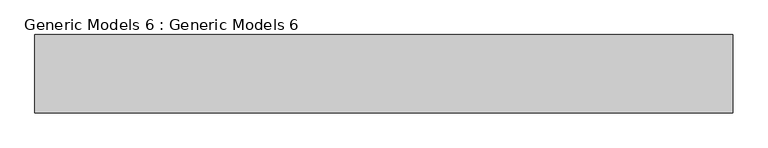
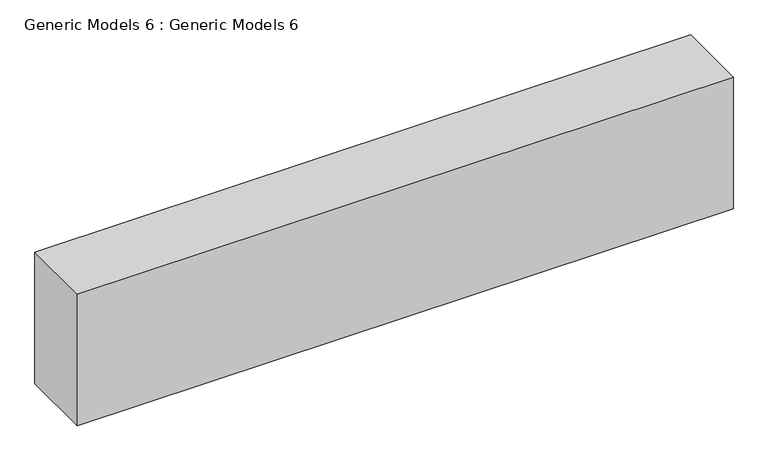
"""IFC4 building model written with IfcOpenShell, lengths in millimetres: proxy geometry, Generic Models 6 : Generic Models 6."""

from ifc_helpers import new_model, si_unit, frame, origin, place, context, project, spatial, polyline, outline, extrude, source, transform, mapped, element, save


def generic_models_6_generic_models_6_7c639092(model_context):
    return source(origin(), model_context, "Body", "SweptSolid", [
        extrude(outline(polyline([(895.326752, -4077.2866303), (-1813.90064, -4077.2866303), (-1813.90064, -3772.4866303), (895.326752, -3772.4866303), (895.326752, -4077.2866303)])), frame((0.0, 0.0, 2988.1285714), z_axis=(0.0, 0.0, 1.0), x_axis=(1.0, 0.0, 0.0)), (0.0, 0.0, 1.0), 575.1285714),
    ])


if __name__ == "__main__":
    model = new_model("IFC4")
    model_context = context("Model", 3, world=origin())
    ifc_project = project(units=[si_unit("LENGTHUNIT", "METRE", prefix="MILLI")], contexts=[model_context])
    site = spatial("IfcSite", under=ifc_project)
    building = spatial("IfcBuilding", under=site)
    placement = place(None, origin())
    generic_models_6_generic_models_6_shape = generic_models_6_generic_models_6_7c639092(model_context)
    element("IfcBuildingElementProxy", 1, Name="Generic Models 6 : Generic Models 6", ObjectType="Generic Models 6 : Generic Models 6", at=placement, inside=building, context=model_context, shape_type="MappedRepresentation", body=[
        mapped(generic_models_6_generic_models_6_shape, transform((0.0, 0.0, 0.0), x_axis=(1.0, 0.0, 0.0), y_axis=(0.0, 1.0, 0.0), z_axis=(0.0, 0.0, 1.0))),
    ])
    save(model, "model.ifc")

# Revit data of these elements
# Element 1 (IfcBuildingElementProxy, "Generic Models 6 : Generic Models 6")
#   Materials on its faces: "Clad - White"
# Materials
#   "Clad - White": class "Wood", colour RGB 242 242 238, transparency 0, Cost = 0
